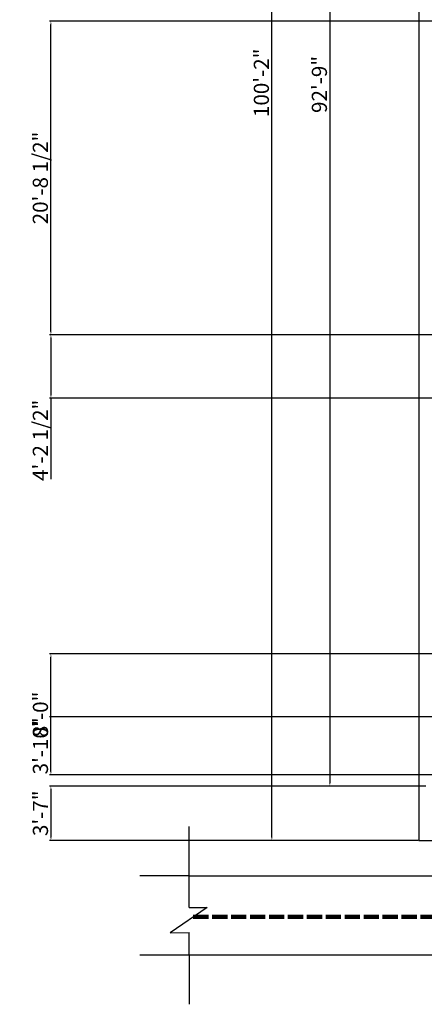
# Model space of a CAD drawing. Units: inches. Extents: x 1947 to 2903, y 1974 to 3472.
# Tile 1 of 5: x 1947 to 2267, y 2055 to 2836. Entities that reach past the tile are written whole.
import ezdxf

# ---------------------------------------------------------------- set-up
doc = ezdxf.new("R2010")
doc.units = ezdxf.units.IN
doc.linetypes.add('ACAD_ISO02W100', pattern=[15, 12, -3])
for name, color, linetype, lineweight in [('A-ANNO-DIMS', 2, 'Continuous', 18), ('C-PROP', 1, 'Continuous', 25), ('C-ROAD', 7, 'Continuous', 25), ('C-ROAD-CNTR', 2, 'ACAD_ISO02W100', 100)]:
    doc.layers.add(name, color=color, linetype=linetype, lineweight=lineweight)
doc.styles.get("Standard").update_dxf_attribs({"font": 'arial.ttf'})
doc.dimstyles.new('ISO-25', dxfattribs={"dimtxt": 12, "dimasz": 2.5, "dimexe": 1.25, "dimexo": 0.625, "dimtad": 1, "dimdec": 0, "dimlunit": 4, "dimtxsty": 'Standard', "dimcen": 2.5, "dimadec": 0, "dimazin": 0, "dimtfac": 1, "dimtdec": 0, "dimtmove": 0, "dimatfit": 3, "dimfxl": 1, "dimarcsym": 0})

# ---------------------------------------------------------------- blocks, each defined once
blk = doc.blocks.new('*D6')
at = {"layer": 'A-ANNO-DIMS', "color": 0, "lineweight": -2, "transparency": 16777216}
for p, q in [((2268.49, 3341.41), (2191.31, 3341.41)), ((2192.56, 3338.91), (2192.56, 2230.91)), ((2268.49, 2228.41), (2191.31, 2228.41))]:
    blk.add_line(p, q, dxfattribs=at)
at = {"layer": 'A-ANNO-DIMS', "color": 0, "lineweight": 100, "transparency": 16777216}
for points in [[(2192.15, 3338.91), (2192.98, 3338.91), (2192.56, 3341.41)], [(2192.15, 2230.91), (2192.98, 2230.91), (2192.56, 2228.41)]]:
    blk.add_solid(points, dxfattribs=at)
at = {"layer": 'Defpoints', "color": 0, "lineweight": 100, "transparency": 16777216}
for p in [(2269.11, 3341.41), (2192.56, 2228.41), (2269.11, 2228.41)]:
    blk.add_point(p, dxfattribs=at)
at = {"layer": 'A-ANNO-DIMS', "color": 0, "transparency": 16777216, "insert": (2185.81, 2784.91), "char_height": 12, "attachment_point": 5, "rotation": 90}
blk.add_mtext('92\'-9"', dxfattribs=at)
blk = doc.blocks.new('*D8')
at = {"layer": 'A-ANNO-DIMS', "color": 0, "lineweight": -2, "transparency": 16777216}
for p, q in [((2262.49, 3386.97), (2145.36, 3386.97)), ((2146.61, 2187.91), (2146.61, 3384.47)), ((2262.49, 2185.41), (2145.36, 2185.41))]:
    blk.add_line(p, q, dxfattribs=at)
at = {"layer": 'A-ANNO-DIMS', "color": 0, "lineweight": 100, "transparency": 16777216}
for points in [[(2146.19, 3384.47), (2147.03, 3384.47), (2146.61, 3386.97)], [(2146.19, 2187.91), (2147.03, 2187.91), (2146.61, 2185.41)]]:
    blk.add_solid(points, dxfattribs=at)
at = {"layer": 'Defpoints', "color": 0, "lineweight": 100, "transparency": 16777216}
for p in [(2146.61, 3386.97), (2263.11, 3386.97), (2263.11, 2185.41)]:
    blk.add_point(p, dxfattribs=at)
at = {"layer": 'A-ANNO-DIMS', "color": 0, "transparency": 16777216, "insert": (2139.86, 2786.19), "char_height": 12, "attachment_point": 5, "rotation": 90}
blk.add_mtext('100\'-2"', dxfattribs=at)
blk = doc.blocks.new('*D34')
at = {"layer": 'A-ANNO-DIMS', "color": 0, "lineweight": -2, "transparency": 16777216}
for p, q in [((2268.49, 2228.41), (1970.32, 2228.41)), ((1971.57, 2225.91), (1971.57, 2187.91)), ((2262.49, 2185.41), (1970.32, 2185.41))]:
    blk.add_line(p, q, dxfattribs=at)
at = {"layer": 'A-ANNO-DIMS', "color": 0, "lineweight": 100, "transparency": 16777216}
for points in [[(1971.16, 2225.91), (1971.99, 2225.91), (1971.57, 2228.41)], [(1971.16, 2187.91), (1971.99, 2187.91), (1971.57, 2185.41)]]:
    blk.add_solid(points, dxfattribs=at)
at = {"layer": 'Defpoints', "color": 0, "lineweight": 100, "transparency": 16777216}
for p in [(2269.11, 2228.41), (1971.57, 2185.41), (2263.11, 2185.41)]:
    blk.add_point(p, dxfattribs=at)
at = {"layer": 'A-ANNO-DIMS', "color": 0, "transparency": 16777216, "insert": (1964.82, 2206.91), "char_height": 12, "attachment_point": 5, "rotation": 90}
blk.add_mtext('3\'-7"', dxfattribs=at)
blk = doc.blocks.new('*D35')
at = {"layer": 'A-ANNO-DIMS', "color": 0, "lineweight": -2, "transparency": 16777216}
for p, q in [((2277.49, 2333.22), (1970.32, 2333.22)), ((1971.57, 2239.91), (1971.57, 2330.72)), ((2277.49, 2237.41), (1970.32, 2237.41))]:
    blk.add_line(p, q, dxfattribs=at)
at = {"layer": 'A-ANNO-DIMS', "color": 0, "lineweight": 100, "transparency": 16777216}
for points in [[(1971.16, 2330.72), (1971.99, 2330.72), (1971.57, 2333.22)], [(1971.16, 2239.91), (1971.99, 2239.91), (1971.57, 2237.41)]]:
    blk.add_solid(points, dxfattribs=at)
at = {"layer": 'Defpoints', "color": 0, "lineweight": 100, "transparency": 16777216}
for p in [(1971.57, 2333.22), (2278.11, 2333.22), (2278.11, 2237.41)]:
    blk.add_point(p, dxfattribs=at)
at = {"layer": 'A-ANNO-DIMS', "color": 0, "transparency": 16777216, "insert": (1964.82, 2285.31), "char_height": 12, "attachment_point": 5, "rotation": 90}
blk.add_mtext('8\'-0"', dxfattribs=at)
blk = doc.blocks.new('*D38')
at = {"layer": 'A-ANNO-DIMS', "color": 0, "lineweight": -2, "transparency": 16777216}
for p, q in [((2277.49, 2835.06), (1970.32, 2835.06)), ((1971.57, 2588.89), (1971.57, 2832.56)), ((2277.49, 2586.39), (1970.32, 2586.39))]:
    blk.add_line(p, q, dxfattribs=at)
at = {"layer": 'A-ANNO-DIMS', "color": 0, "lineweight": 100, "transparency": 16777216}
for points in [[(1971.16, 2832.56), (1971.99, 2832.56), (1971.57, 2835.06)], [(1971.16, 2588.89), (1971.99, 2588.89), (1971.57, 2586.39)]]:
    blk.add_solid(points, dxfattribs=at)
at = {"layer": 'Defpoints', "color": 0, "lineweight": 100, "transparency": 16777216}
for p in [(1971.57, 2835.06), (2278.11, 2835.06), (2278.11, 2586.39)]:
    blk.add_point(p, dxfattribs=at)
at = {"layer": 'A-ANNO-DIMS', "color": 0, "transparency": 16777216, "insert": (1964.74, 2710.73), "char_height": 12, "attachment_point": 5, "rotation": 90}
blk.add_mtext('20\'-8 1/2"', dxfattribs=at)
blk = doc.blocks.new('*D44')
at = {"layer": 'A-ANNO-DIMS', "color": 0, "lineweight": -2, "transparency": 16777216}
for p, q in [((2569.57, 2283.31), (1970.32, 2283.31)), ((1971.57, 2239.91), (1971.57, 2280.81)), ((2569.57, 2237.41), (1970.32, 2237.41))]:
    blk.add_line(p, q, dxfattribs=at)
at = {"layer": 'A-ANNO-DIMS', "color": 0, "lineweight": 100, "transparency": 16777216}
for points in [[(1971.16, 2280.81), (1971.99, 2280.81), (1971.57, 2283.31)], [(1971.16, 2239.91), (1971.99, 2239.91), (1971.57, 2237.41)]]:
    blk.add_solid(points, dxfattribs=at)
at = {"layer": 'Defpoints', "color": 0, "lineweight": 100, "transparency": 16777216}
for p in [(1971.57, 2283.31), (2570.2, 2283.31), (2570.2, 2237.41)]:
    blk.add_point(p, dxfattribs=at)
at = {"layer": 'A-ANNO-DIMS', "color": 0, "transparency": 16777216, "insert": (1964.82, 2260.36), "char_height": 12, "attachment_point": 5, "rotation": 90}
blk.add_mtext('3\'-10"', dxfattribs=at)
blk = doc.blocks.new('*D45')
at = {"layer": 'A-ANNO-DIMS', "color": 0, "lineweight": -2, "transparency": 16777216}
for p, q in [((2277.49, 2586.39), (1970.32, 2586.39)), ((1971.57, 2583.89), (1971.57, 2538.49)), ((2277.49, 2535.99), (1970.32, 2535.99)), ((1971.57, 2535.99), (1971.57, 2471.89))]:
    blk.add_line(p, q, dxfattribs=at)
at = {"layer": 'A-ANNO-DIMS', "color": 0, "lineweight": 100, "transparency": 16777216}
for points in [[(1971.16, 2583.89), (1971.99, 2583.89), (1971.57, 2586.39)], [(1971.16, 2538.49), (1971.99, 2538.49), (1971.57, 2535.99)]]:
    blk.add_solid(points, dxfattribs=at)
at = {"layer": 'Defpoints', "color": 0, "lineweight": 100, "transparency": 16777216}
for p in [(2278.11, 2586.39), (1971.57, 2535.99), (2278.11, 2535.99)]:
    blk.add_point(p, dxfattribs=at)
at = {"layer": 'A-ANNO-DIMS', "color": 0, "transparency": 16777216, "insert": (1964.74, 2502.69), "char_height": 12, "attachment_point": 5, "rotation": 90}
blk.add_mtext('4\'-2 1/2"', dxfattribs=at)

msp = doc.modelspace()

# ---------------------------------------------------------------- linework, layer by layer
at = {"layer": 'C-PROP'}
for p, q in [((2263.11, 3341.41), (2263.11, 2228.41)), ((2263.11, 2228.41), (2263.11, 2185.41)), ((2263.11, 2189.41), (2263.11, 2187.41)), ((2263.11, 2185.41), (2743.11, 2185.41))]:
    msp.add_line(p, q, dxfattribs=at)
at = {"layer": 'C-ROAD'}
for p, q in [((2081.02, 2157.31), (2081.02, 2196.31)), ((2081.02, 2157.31), (2042.1, 2157.31)), ((2095.32, 2132.17), (2066.04, 2112.15)), ((2081.02, 2132.17), (2095.32, 2132.17)), ((2066.04, 2112.15), (2081.02, 2112.46)), ((2081.02, 2094.4), (2042.02, 2094.4)), ((2081.02, 2094.4), (2081.02, 2055.4))]:
    msp.add_line(p, q, dxfattribs=at)
for points in [[(2081.02, 2132.17), (2081.02, 2157.31), (2792.52, 2157.31), (2792.52, 2134.53)], [(2792.52, 2114.81), (2792.52, 2094.4), (2081.02, 2094.4), (2081.02, 2112.46)]]:
    msp.add_lwpolyline(points, dxfattribs=at)
at = {"layer": 'C-ROAD-CNTR'}
msp.add_line((2084.35, 2124.67), (2792.4, 2124.67), dxfattribs=at)

# ---------------------------------------------------------------- dimensions: what is measured, and where the dimension line sits
at = {"layer": 'A-ANNO-DIMS'}
for base, p1, p2, override, picture, middle in [((2146.61, 3386.97), (2263.11, 2185.41), (2263.11, 3386.97), {"dimclrd": 0, "dimclre": 0, "dimclrt": 0}, '*D8', (2139.86, 2786.19)), ((2192.56, 2228.41), (2269.11, 3341.41), (2269.11, 2228.41), {"dimclrd": 0, "dimclre": 0, "dimclrt": 0}, '*D6', (2185.81, 2784.91)), ((1971.57, 2835.06), (2278.11, 2586.39), (2278.11, 2835.06), {"dimdec": 1, "dimlfac": 1, "dimrnd": 0, "dimzin": 1, "dimdsep": 46, "dimlunit": 4, "dimfrac": 2}, '*D38', (1964.74, 2710.73)), ((1971.57, 2535.99), (2278.11, 2586.39), (2278.11, 2535.99), {"dimdec": 1, "dimlfac": 1, "dimrnd": 0, "dimzin": 1, "dimdsep": 46, "dimlunit": 4, "dimfrac": 2}, '*D45', (1964.74, 2502.69)), ((1971.57, 2333.22), (2278.11, 2237.41), (2278.11, 2333.22), {"dimdec": 1, "dimlfac": 1, "dimrnd": 0, "dimzin": 1, "dimdsep": 46, "dimlunit": 4, "dimfrac": 2}, '*D35', (1964.82, 2285.31)), ((1971.57, 2283.31), (2570.2, 2237.41), (2570.2, 2283.31), {"dimdec": 1, "dimlfac": 1, "dimrnd": 0, "dimzin": 1, "dimdsep": 46, "dimlunit": 4, "dimfrac": 2}, '*D44', (1964.82, 2260.36)), ((1971.57, 2185.41), (2269.11, 2228.41), (2263.11, 2185.41), {"dimdec": 1, "dimlfac": 1, "dimrnd": 0, "dimzin": 1, "dimdsep": 46, "dimlunit": 4, "dimfrac": 2}, '*D34', (1964.82, 2206.91))]:
    dim = msp.add_linear_dim(base=base, p1=p1, p2=p2, angle=90, dimstyle='ISO-25', override=override, dxfattribs=at)
    dim.commit()
    dim.dimension.update_dxf_attribs({"geometry": picture, "text_midpoint": middle})

doc.saveas('drawing.dxf')
